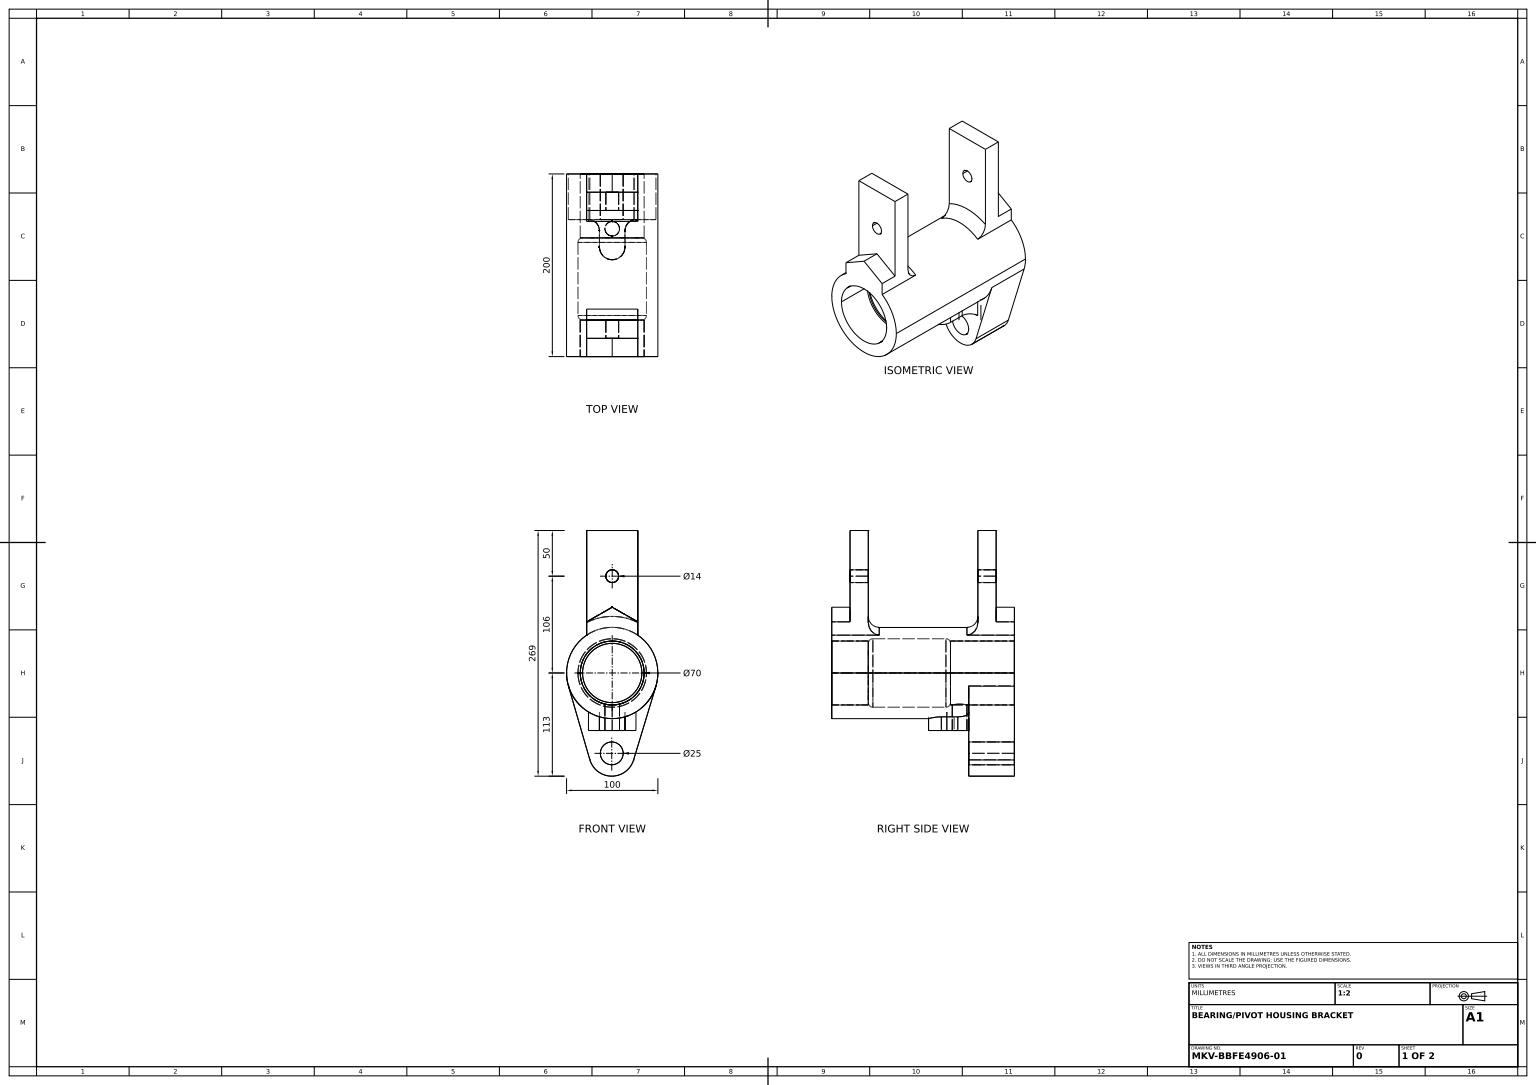
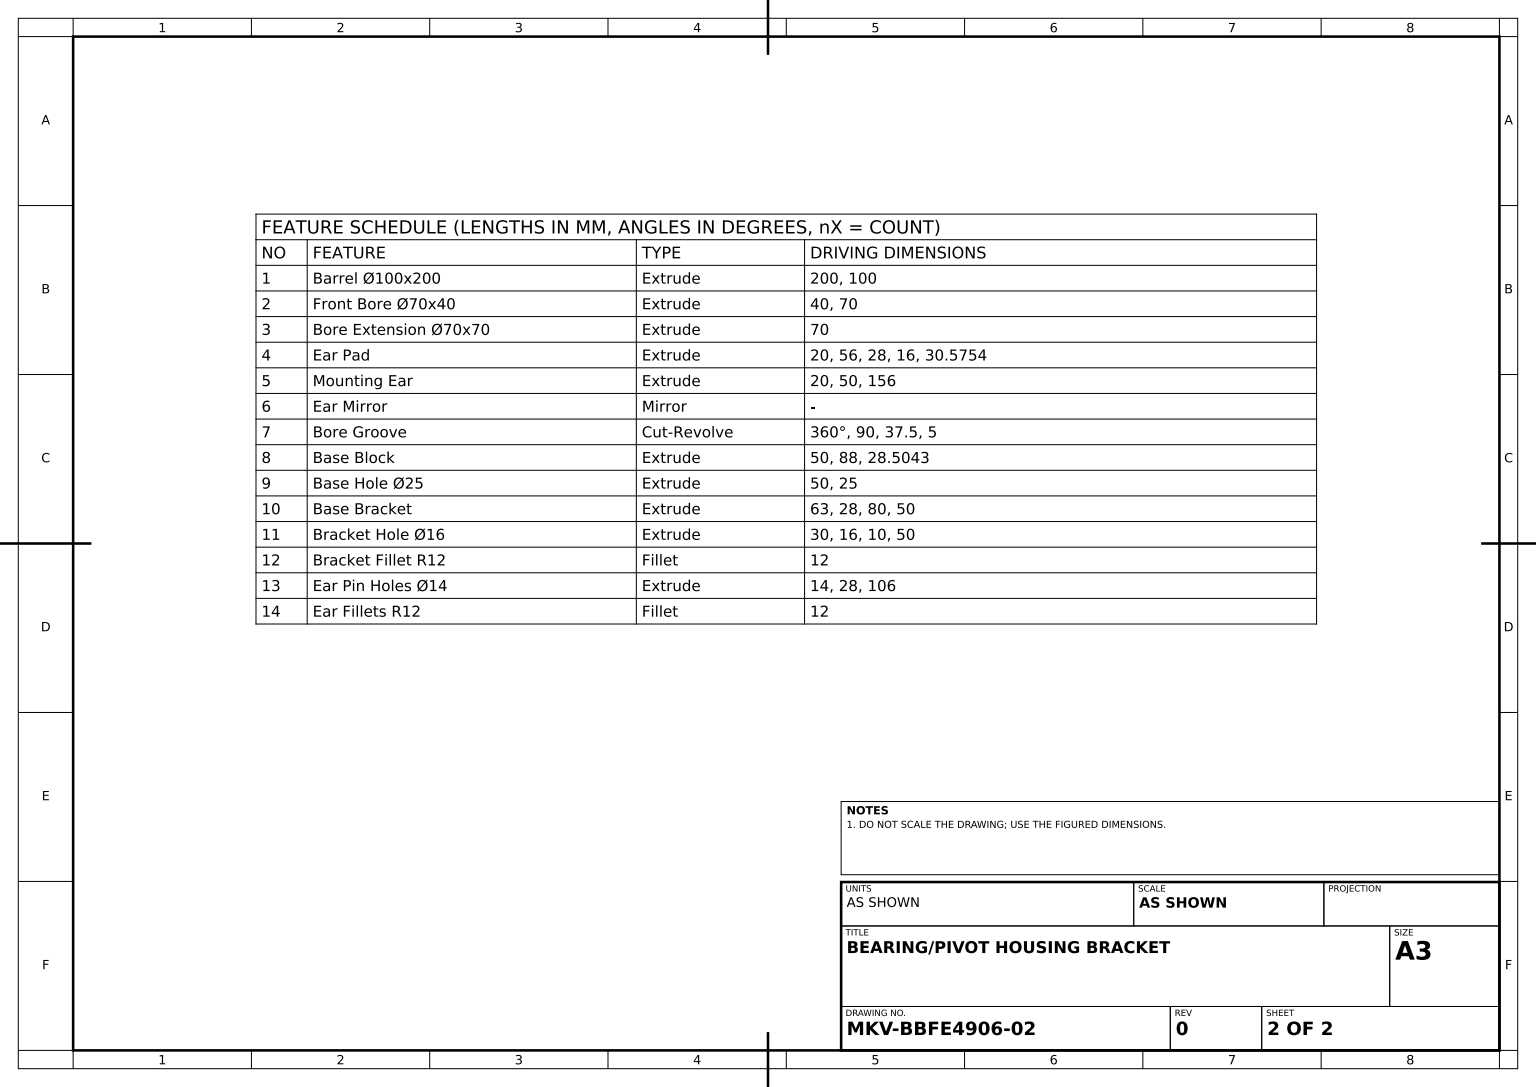
from build123d import *

# Parameters (mm, degrees)
BARREL_PROFILE_100_R       = 50
BARREL_100X200_DEPTH       = 200
FRONT_BORE_PROFILE_70_R    = 35
FRONT_BORE_70X40_DEPTH     = 40
BORE_START                 = -70
BORE_EXTENSION_PROFILE_R   = 35
BORE_EXTENSION_70X70_DEPTH = 70
EAR_PAD_DEPTH              = 20
MOUNTING_EAR_DEPTH         = 20
BASE_START                 = -50
BASE_BLOCK_DEPTH           = 50
BASE_HOLE_PROFILE_25_R     = 12.5
BASE_HOLE_25_DEPTH         = 50
BASE_BRACKET_REACH         = 302.767
BASE_BRACKET_END_RADIUS    = 50
BRACKET_HOLE_PROFILE_16_R  = 8
BRACKET_HOLE_16_DEPTH      = 30
BRACKET_FILLET_R12_R       = 12
EAR_PIN_HOLE_PROFILE_14_R  = 7
EAR_PIN_HOLES_14_DEPTH     = 244.384469607
EAR_FILLETS_R12_R          = 12


with BuildPart() as part:
    # Barrel Profile Ø100 → Barrel Ø100x200 (new body)
    with BuildSketch(Plane.XY):
        Circle(BARREL_PROFILE_100_R)
    extrude(amount=-BARREL_100X200_DEPTH)

    # Front Bore Profile Ø70 → Front Bore Ø70x40 (cut)
    with BuildSketch(Plane.XY):
        Circle(FRONT_BORE_PROFILE_70_R)
    extrude(amount=-FRONT_BORE_70X40_DEPTH, mode=Mode.SUBTRACT)

    # Bore Extension Profile → Bore Extension Ø70x70 (cut)
    with BuildSketch(Plane(origin=(0, 0, -200), x_dir=(-1, 0, 0), z_dir=(0, 0, -1)).offset(BORE_START)):
        with Locations(Location((0, 0, 0), (0, 0, 180))):
            Circle(BORE_EXTENSION_PROFILE_R)
    extrude(amount=BORE_EXTENSION_70X70_DEPTH, mode=Mode.SUBTRACT)

    # Ear Pad Profile → Ear Pad (add)
    with BuildSketch(Plane.XY):
        with BuildLine():
            Line((-28, 41.424630354), (-28, 56))
            Line((-28, 56), (0, 72))
            Line((0, 72), (28, 56))
            Line((28, 56), (28, 41.424630354))
            ThreePointArc((28, 41.424630354), (0, 50), (-28, 41.424630354))
        make_face()
    ear_pad = extrude(amount=-EAR_PAD_DEPTH)

    # Ear Profile → Mounting Ear (add)
    with BuildSketch(Plane(origin=(0, 0, -20), x_dir=(-1, 0, 0), z_dir=(0, 0, -1))):
        with BuildLine():
            Line((-28, 41.424630354), (-28, 56))
            Line((-28, 56), (-28, 156))
            Line((-28, 156), (28, 156))
            Line((28, 156), (28, 41.424630354))
            ThreePointArc((28, 41.424630354), (0, 50), (-28, 41.424630354))
        make_face()
    mounting_ear = extrude(amount=MOUNTING_EAR_DEPTH)

    # Ear Mirror: Ear Pad, Mounting Ear across plane
    add(ear_pad.mirror(Plane.XY.offset(-100)))
    add(mounting_ear.mirror(Plane.XY.offset(-100)))

    # Bore Groove Profile → Bore Groove (revolve, cut)
    with BuildSketch(Plane(origin=(0, 0, 0), x_dir=(0, 0, -1), z_dir=(1, 0, 0)), mode=Mode.PRIVATE) as bore_groove_sk:
        with BuildLine():
            Line((40, 0), (40, 32.5))
            ThreePointArc((40, 32.5), (41.464466094, 36.035533906), (45, 37.5))
            Line((45, 37.5), (125, 37.5))
            ThreePointArc((125, 37.5), (128.535533906, 36.035533906), (130, 32.5))
            Line((130, 32.5), (130, 0))
            Line((130, 0), (40, 0))
        make_face()
    revolve(bore_groove_sk.sketch.rotate(Axis((0, 0, -40), (0, 0, -1)), 90), axis=Axis((0, 0, -40), (0, 0, -1)), mode=Mode.SUBTRACT)

    # Base Block Profile → Base Block (add)
    with BuildSketch(Plane(origin=(0, 0, -200), x_dir=(-1, 0, 0), z_dir=(0, 0, -1)).offset(BASE_START)):
        with BuildLine():
            Line((-23.424549882, -95.238072549), (-47.857680112, -14.479034992))
            ThreePointArc((-47.857680112, -14.479034992), (0.286528508, -49.999179007), (48.020480401, -13.929589444))
            Line((48.020480401, -13.929589444), (24.514530374, -94.963349775))
            ThreePointArc((24.514530374, -94.963349775), (0.647554428, -112.998144557), (-23.424549882, -95.238072549))
        make_face()
    extrude(amount=BASE_BLOCK_DEPTH)

    # Base Hole Profile Ø25 → Base Hole Ø25 (cut)
    with BuildSketch(Plane.XY.offset(-150)):
        with Locations((-0.504290174, -87.998555053)):
            Circle(BASE_HOLE_PROFILE_25_R)
    extrude(amount=-BASE_HOLE_25_DEPTH, mode=Mode.SUBTRACT)

    # Base Bracket: up to this cylinder (the profile starts outside it)
    base_bracket_end = Plane(origin=(0, 0, -129.383127), z_dir=(0, 0, 1)) * Cylinder(BASE_BRACKET_END_RADIUS, 706.534, mode=Mode.PRIVATE)
    # Base Bracket Profile → Base Bracket (add, up to the surface)
    with BuildSketch(Plane(origin=(0, -63, 0), x_dir=(1, 0, 0), z_dir=(0, 1, 0)), mode=Mode.PRIVATE) as base_bracket_sk1:
        with BuildLine():
            Line((-14, 120), (-14, 150))
            Line((-14, 150), (14, 150))
            Line((14, 150), (14, 120))
            ThreePointArc((14, 120), (0, 106), (-14, 120))
        make_face()
    base_bracket_tool1 = extrude(base_bracket_sk1.sketch, amount=BASE_BRACKET_REACH, mode=Mode.PRIVATE) - base_bracket_end
    add(base_bracket_tool1.solids().sort_by_distance((0, -63, -129.383127))[0])

    # Bracket Hole Profile Ø16 → Bracket Hole Ø16 (cut)
    with BuildSketch(Plane.XZ.offset(63)):
        with Locations(Location((0, -140, 0), (0, 0, 270))):
            Circle(BRACKET_HOLE_PROFILE_16_R)
    extrude(amount=-BRACKET_HOLE_16_DEPTH, mode=Mode.SUBTRACT)

    # Bracket Fillet R12
    bracket_fillet_r12_edges = [part.edges().sort_by_distance(p)[0] for p in [
        (-14, -55.5, -150),
        (14, -55.5, -150),
    ]]
    fillet(bracket_fillet_r12_edges, radius=BRACKET_FILLET_R12_R)

    # Ear Pin Hole Profile Ø14 → Ear Pin Holes Ø14 (cut, through all)
    with BuildSketch(Plane.XY.offset(-20)):
        with Locations((0, 106)):
            Circle(EAR_PIN_HOLE_PROFILE_14_R)
    extrude(amount=-EAR_PIN_HOLES_14_DEPTH, mode=Mode.SUBTRACT)

    # Ear Fillets R12
    ear_fillets_r12_edges = [part.edges().sort_by_distance(p)[0] for p in [
        (0, 50, -40),
        (0, 50, -160),
    ]]
    fillet(ear_fillets_r12_edges, radius=EAR_FILLETS_R12_R)


solid = part.part
